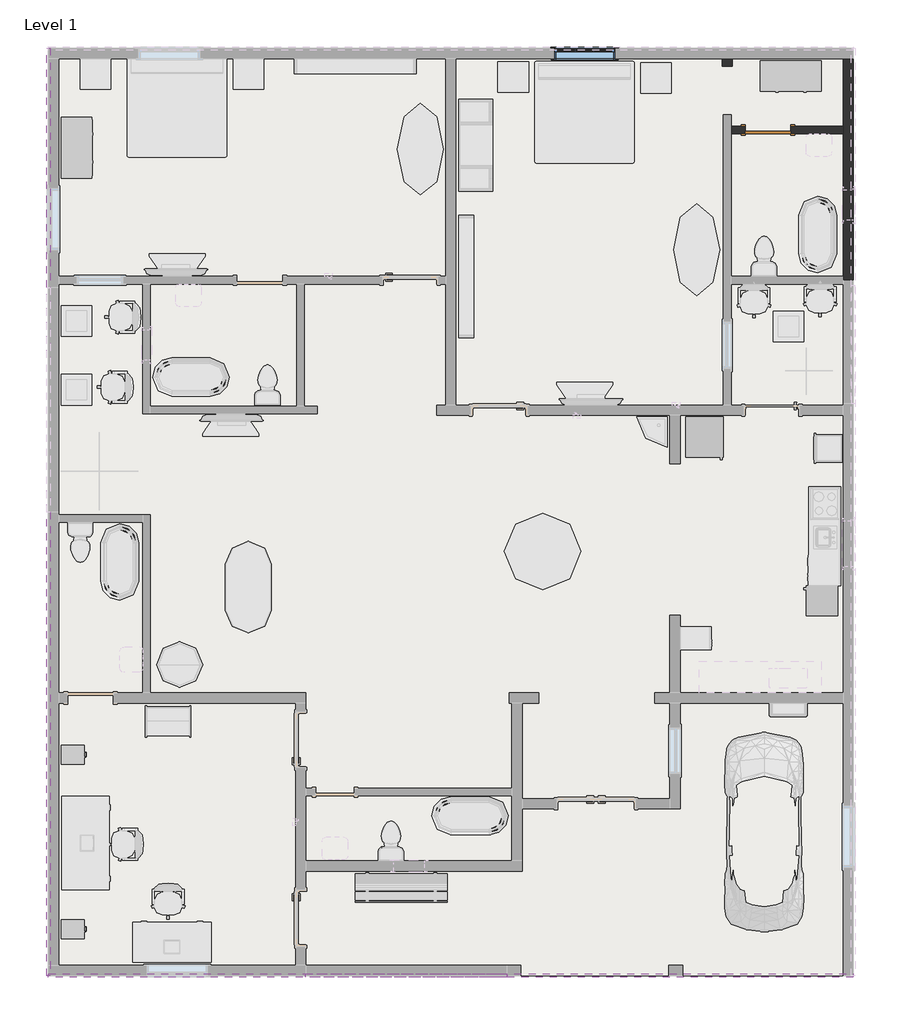
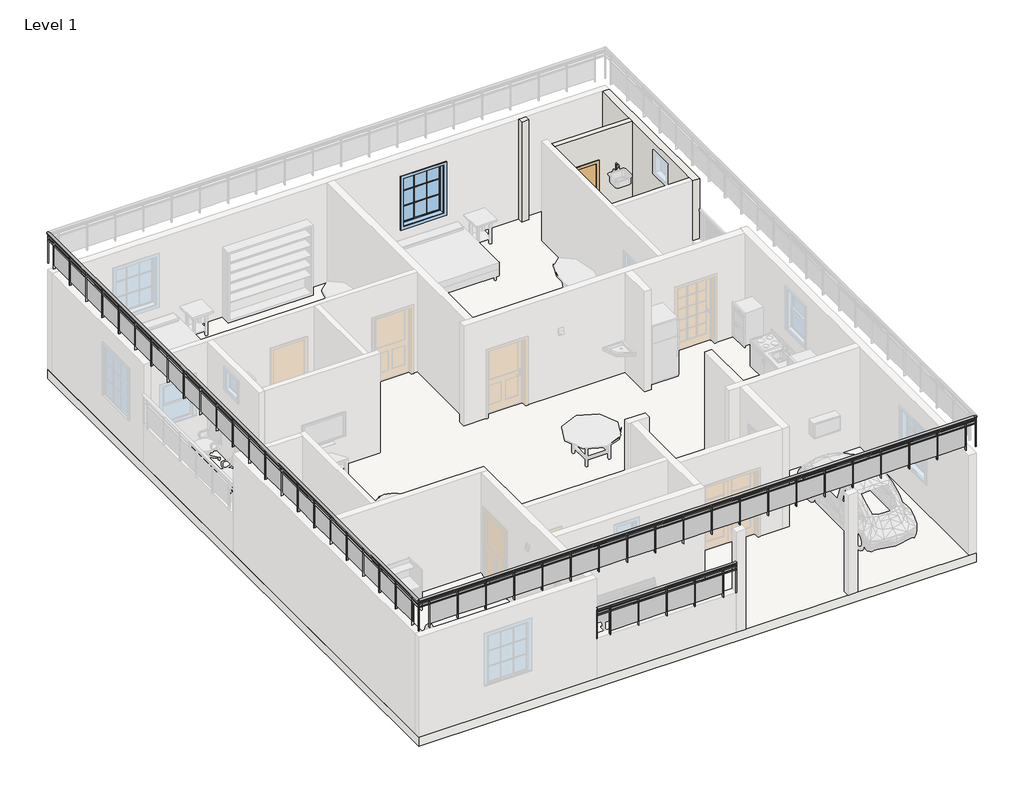
# One storey, part 2 of 4: 3 railings, 3 walls, 1 door, 1 slab, 1 window.
"""IFC4 building model written with IfcOpenShell, lengths in millimetres."""

from ifc_helpers import new_model, si_unit, point, frame, origin, origin_with_axes, place, context, project, spatial, polyline, ellipse_curve, trimmed, outline, extrude, faceted_brep, transform, mapped, element, save
from ifc_brep_helpers import plane_surface, extruded_surface, advanced_brep
from components import door_16372e1c, window_cfa1ffdd

model = new_model("IFC4")

# Units and contexts
model_context = context("Model", 3, world=origin())
ifc_project = project(units=[si_unit("LENGTHUNIT", "METRE", prefix="MILLI")], contexts=[model_context])

# Site, building, storey
site = spatial("IfcSite", under=ifc_project)
building = spatial("IfcBuilding", under=site)
storey = spatial("IfcBuildingStorey", under=building, Name="Level 1", Elevation=0.0)

# Door
placement = place(None, origin())
door_shape = door_16372e1c(model_context)
element("IfcDoor", 1, ObjectType="Single-Flush : 36\" x 84\"", at=placement, inside=storey, context=model_context, shape_type="MappedRepresentation", body=[
    mapped(door_shape, transform((-3290.7484731, 10947.0442281, 0.0), x_axis=(-1.0, 0.0, 0.0), y_axis=(0.0, -1.0, 0.0), z_axis=(0.0, 0.0, 1.0))),
])

# Railings
element("IfcRailing", 2, ObjectType="Glass Panel - Bottom Fill", at=placement, inside=storey, context=model_context, shape_type="SolidModel", body=[
    advanced_brep(
    [(-17603.6484731, 12572.6442281, 4165.6), (-17679.8484731, 12572.6442281, 4165.6), (-17603.6484731, -5918.5557719, 4165.6), (-17679.8484731, -5918.5557719, 4165.6)],
    [
        (0, 1, ellipse_curve(frame((-17641.7484731, 12572.6442281, 4165.6), z_axis=(0.0, 1.0, 0.0), x_axis=(-1.0, 0.0, 0.0)), 38.1, 28.575)),
        (1, 0, ellipse_curve(frame((-17641.7484731, 12572.6442281, 4165.6), z_axis=(0.0, 1.0, 0.0), x_axis=(-1.0, 0.0, 0.0)), 38.1, 28.575)),
        (2, 3, ellipse_curve(frame((-17641.7484731, -5918.5557719, 4165.6), z_axis=(0.0, -1.0, 0.0), x_axis=(-1.0, 0.0, 0.0)), 38.1, 28.575)),
        (3, 2, ellipse_curve(frame((-17641.7484731, -5918.5557719, 4165.6), z_axis=(0.0, -1.0, 0.0), x_axis=(-1.0, 0.0, 0.0)), 38.1, 28.575)),
        (0, 2),
        (3, 1),
    ],
    [
        plane_surface(frame((-17641.7484731, 12572.6442281, 4165.6), z_axis=(0.0, 1.0, 0.0), x_axis=(0.0, 0.0, -1.0))),
        plane_surface(frame((-17641.7484731, -5918.5557719, 4165.6), z_axis=(0.0, -1.0, 0.0), x_axis=(0.0, 0.0, -1.0))),
        extruded_surface(trimmed(ellipse_curve(frame((-17641.7484731, -5918.5557719, 4165.6), z_axis=(0.0, 1.0, 0.0), x_axis=(-1.0, 0.0, 0.0)), 38.1, 28.575), [point((-17603.6484731, -5918.5557719, 4165.6))], [point((-17679.8484731, -5918.5557719, 4165.6))], True, "CARTESIAN"), (0.0, 18491.2, 0.0), 18491.2),
        extruded_surface(trimmed(ellipse_curve(frame((-17641.7484731, -5918.5557719, 4165.6), z_axis=(0.0, 1.0, 0.0), x_axis=(-1.0, 0.0, 0.0)), 38.1, 28.575), [point((-17679.8484731, -5918.5557719, 4165.6))], [point((-17603.6484731, -5918.5557719, 4165.6))], True, "CARTESIAN"), (0.0, 18491.2, 0.0), 18491.2),
    ],
    [
        (0, [[1, 2]]),
        (1, [[3, 4]]),
        (2, [[-1, 5, -4, 6]]),
        (3, [[-2, -6, -3, -5]]),
    ],
),
    extrude(outline(polyline([(-17654.4484731, 12572.6442281), (-17629.0484731, 12572.6442281), (-17629.0484731, -5918.5557719), (-17654.4484731, -5918.5557719), (-17654.4484731, 12572.6442281)])), frame((0.0, 0.0, 4051.3), z_axis=(0.0, 0.0, 1.0), x_axis=(1.0, 0.0, 0.0)), (0.0, 0.0, 1.0), 25.4),
    extrude(outline(polyline([(-17654.4484731, 12572.6442281), (-17629.0484731, 12572.6442281), (-17629.0484731, -5918.5557719), (-17654.4484731, -5918.5557719), (-17654.4484731, 12572.6442281)])), frame((0.0, 0.0, 3949.7), z_axis=(0.0, 0.0, 1.0), x_axis=(1.0, 0.0, 0.0)), (0.0, 0.0, 1.0), 25.4),
    extrude(outline(polyline([(-17667.1484731, -5607.4057719), (-17616.3484731, -5607.4057719), (-17616.3484731, -5620.1057719), (-17667.1484731, -5620.1057719), (-17667.1484731, -5607.4057719)])), frame((0.0, 0.0, 3251.2), z_axis=(0.0, 0.0, 1.0), x_axis=(1.0, 0.0, 0.0)), (0.0, 0.0, 1.0), 885.6788223),
    extrude(outline(polyline([(-17635.2133161, -4800.9557719), (-17635.2133161, -5613.7557719), (-17641.5633161, -5613.7557719), (-17641.5633161, -4800.9557719), (-17635.2133161, -4800.9557719)])), frame((0.0, 0.0, 3352.8), z_axis=(0.0, 0.0, 1.0), x_axis=(1.0, 0.0, 0.0)), (0.0, 0.0, 1.0), 596.9),
    extrude(outline(polyline([(-17667.1484731, -4794.6057719), (-17616.3484731, -4794.6057719), (-17616.3484731, -4807.3057719), (-17667.1484731, -4807.3057719), (-17667.1484731, -4794.6057719)])), frame((0.0, 0.0, 3251.2), z_axis=(0.0, 0.0, 1.0), x_axis=(1.0, 0.0, 0.0)), (0.0, 0.0, 1.0), 885.6788223),
    extrude(outline(polyline([(-17635.2133161, -3988.1557719), (-17635.2133161, -4800.9557719), (-17641.5633161, -4800.9557719), (-17641.5633161, -3988.1557719), (-17635.2133161, -3988.1557719)])), frame((0.0, 0.0, 3352.8), z_axis=(0.0, 0.0, 1.0), x_axis=(1.0, 0.0, 0.0)), (0.0, 0.0, 1.0), 596.9),
    extrude(outline(polyline([(-17667.1484731, -3981.8057719), (-17616.3484731, -3981.8057719), (-17616.3484731, -3994.5057719), (-17667.1484731, -3994.5057719), (-17667.1484731, -3981.8057719)])), frame((0.0, 0.0, 3251.2), z_axis=(0.0, 0.0, 1.0), x_axis=(1.0, 0.0, 0.0)), (0.0, 0.0, 1.0), 885.6788223),
    extrude(outline(polyline([(-17635.2133161, -3175.3557719), (-17635.2133161, -3988.1557719), (-17641.5633161, -3988.1557719), (-17641.5633161, -3175.3557719), (-17635.2133161, -3175.3557719)])), frame((0.0, 0.0, 3352.8), z_axis=(0.0, 0.0, 1.0), x_axis=(1.0, 0.0, 0.0)), (0.0, 0.0, 1.0), 596.9),
    extrude(outline(polyline([(-17667.1484731, -3169.0057719), (-17616.3484731, -3169.0057719), (-17616.3484731, -3181.7057719), (-17667.1484731, -3181.7057719), (-17667.1484731, -3169.0057719)])), frame((0.0, 0.0, 3251.2), z_axis=(0.0, 0.0, 1.0), x_axis=(1.0, 0.0, 0.0)), (0.0, 0.0, 1.0), 885.6788223),
    extrude(outline(polyline([(-17635.2133161, -2362.5557719), (-17635.2133161, -3175.3557719), (-17641.5633161, -3175.3557719), (-17641.5633161, -2362.5557719), (-17635.2133161, -2362.5557719)])), frame((0.0, 0.0, 3352.8), z_axis=(0.0, 0.0, 1.0), x_axis=(1.0, 0.0, 0.0)), (0.0, 0.0, 1.0), 596.9),
    extrude(outline(polyline([(-17667.1484731, -2356.2057719), (-17616.3484731, -2356.2057719), (-17616.3484731, -2368.9057719), (-17667.1484731, -2368.9057719), (-17667.1484731, -2356.2057719)])), frame((0.0, 0.0, 3251.2), z_axis=(0.0, 0.0, 1.0), x_axis=(1.0, 0.0, 0.0)), (0.0, 0.0, 1.0), 885.6788223),
    extrude(outline(polyline([(-17635.2133161, -1549.7557719), (-17635.2133161, -2362.5557719), (-17641.5633161, -2362.5557719), (-17641.5633161, -1549.7557719), (-17635.2133161, -1549.7557719)])), frame((0.0, 0.0, 3352.8), z_axis=(0.0, 0.0, 1.0), x_axis=(1.0, 0.0, 0.0)), (0.0, 0.0, 1.0), 596.9),
    extrude(outline(polyline([(-17667.1484731, -1543.4057719), (-17616.3484731, -1543.4057719), (-17616.3484731, -1556.1057719), (-17667.1484731, -1556.1057719), (-17667.1484731, -1543.4057719)])), frame((0.0, 0.0, 3251.2), z_axis=(0.0, 0.0, 1.0), x_axis=(1.0, 0.0, 0.0)), (0.0, 0.0, 1.0), 885.6788223),
    extrude(outline(polyline([(-17635.2133161, -736.9557719), (-17635.2133161, -1549.7557719), (-17641.5633161, -1549.7557719), (-17641.5633161, -736.9557719), (-17635.2133161, -736.9557719)])), frame((0.0, 0.0, 3352.8), z_axis=(0.0, 0.0, 1.0), x_axis=(1.0, 0.0, 0.0)), (0.0, 0.0, 1.0), 596.9),
    extrude(outline(polyline([(-17667.1484731, -730.6057719), (-17616.3484731, -730.6057719), (-17616.3484731, -743.3057719), (-17667.1484731, -743.3057719), (-17667.1484731, -730.6057719)])), frame((0.0, 0.0, 3251.2), z_axis=(0.0, 0.0, 1.0), x_axis=(1.0, 0.0, 0.0)), (0.0, 0.0, 1.0), 885.6788223),
    extrude(outline(polyline([(-17635.2133161, 75.8442281), (-17635.2133161, -736.9557719), (-17641.5633161, -736.9557719), (-17641.5633161, 75.8442281), (-17635.2133161, 75.8442281)])), frame((0.0, 0.0, 3352.8), z_axis=(0.0, 0.0, 1.0), x_axis=(1.0, 0.0, 0.0)), (0.0, 0.0, 1.0), 596.9),
    extrude(outline(polyline([(-17667.1484731, 82.1942281), (-17616.3484731, 82.1942281), (-17616.3484731, 69.4942281), (-17667.1484731, 69.4942281), (-17667.1484731, 82.1942281)])), frame((0.0, 0.0, 3251.2), z_axis=(0.0, 0.0, 1.0), x_axis=(1.0, 0.0, 0.0)), (0.0, 0.0, 1.0), 885.6788223),
    extrude(outline(polyline([(-17635.2133161, 888.6442281), (-17635.2133161, 75.8442281), (-17641.5633161, 75.8442281), (-17641.5633161, 888.6442281), (-17635.2133161, 888.6442281)])), frame((0.0, 0.0, 3352.8), z_axis=(0.0, 0.0, 1.0), x_axis=(1.0, 0.0, 0.0)), (0.0, 0.0, 1.0), 596.9),
    extrude(outline(polyline([(-17667.1484731, 894.9942281), (-17616.3484731, 894.9942281), (-17616.3484731, 882.2942281), (-17667.1484731, 882.2942281), (-17667.1484731, 894.9942281)])), frame((0.0, 0.0, 3251.2), z_axis=(0.0, 0.0, 1.0), x_axis=(1.0, 0.0, 0.0)), (0.0, 0.0, 1.0), 885.6788223),
    extrude(outline(polyline([(-17635.2133161, 1701.4442281), (-17635.2133161, 888.6442281), (-17641.5633161, 888.6442281), (-17641.5633161, 1701.4442281), (-17635.2133161, 1701.4442281)])), frame((0.0, 0.0, 3352.8), z_axis=(0.0, 0.0, 1.0), x_axis=(1.0, 0.0, 0.0)), (0.0, 0.0, 1.0), 596.9),
    extrude(outline(polyline([(-17667.1484731, 1707.7942281), (-17616.3484731, 1707.7942281), (-17616.3484731, 1695.0942281), (-17667.1484731, 1695.0942281), (-17667.1484731, 1707.7942281)])), frame((0.0, 0.0, 3251.2), z_axis=(0.0, 0.0, 1.0), x_axis=(1.0, 0.0, 0.0)), (0.0, 0.0, 1.0), 885.6788223),
    extrude(outline(polyline([(-17635.2133161, 2514.2442281), (-17635.2133161, 1701.4442281), (-17641.5633161, 1701.4442281), (-17641.5633161, 2514.2442281), (-17635.2133161, 2514.2442281)])), frame((0.0, 0.0, 3352.8), z_axis=(0.0, 0.0, 1.0), x_axis=(1.0, 0.0, 0.0)), (0.0, 0.0, 1.0), 596.9),
    extrude(outline(polyline([(-17667.1484731, 2520.5942281), (-17616.3484731, 2520.5942281), (-17616.3484731, 2507.8942281), (-17667.1484731, 2507.8942281), (-17667.1484731, 2520.5942281)])), frame((0.0, 0.0, 3251.2), z_axis=(0.0, 0.0, 1.0), x_axis=(1.0, 0.0, 0.0)), (0.0, 0.0, 1.0), 885.6788223),
    extrude(outline(polyline([(-17635.2133161, 3327.0442281), (-17635.2133161, 2514.2442281), (-17641.5633161, 2514.2442281), (-17641.5633161, 3327.0442281), (-17635.2133161, 3327.0442281)])), frame((0.0, 0.0, 3352.8), z_axis=(0.0, 0.0, 1.0), x_axis=(1.0, 0.0, 0.0)), (0.0, 0.0, 1.0), 596.9),
    extrude(outline(polyline([(-17667.1484731, 3333.3942281), (-17616.3484731, 3333.3942281), (-17616.3484731, 3320.6942281), (-17667.1484731, 3320.6942281), (-17667.1484731, 3333.3942281)])), frame((0.0, 0.0, 3251.2), z_axis=(0.0, 0.0, 1.0), x_axis=(1.0, 0.0, 0.0)), (0.0, 0.0, 1.0), 885.6788223),
    extrude(outline(polyline([(-17635.2133161, 4139.8442281), (-17635.2133161, 3327.0442281), (-17641.5633161, 3327.0442281), (-17641.5633161, 4139.8442281), (-17635.2133161, 4139.8442281)])), frame((0.0, 0.0, 3352.8), z_axis=(0.0, 0.0, 1.0), x_axis=(1.0, 0.0, 0.0)), (0.0, 0.0, 1.0), 596.9),
    extrude(outline(polyline([(-17667.1484731, 4146.1942281), (-17616.3484731, 4146.1942281), (-17616.3484731, 4133.4942281), (-17667.1484731, 4133.4942281), (-17667.1484731, 4146.1942281)])), frame((0.0, 0.0, 3251.2), z_axis=(0.0, 0.0, 1.0), x_axis=(1.0, 0.0, 0.0)), (0.0, 0.0, 1.0), 885.6788223),
    extrude(outline(polyline([(-17635.2133161, 4952.6442281), (-17635.2133161, 4139.8442281), (-17641.5633161, 4139.8442281), (-17641.5633161, 4952.6442281), (-17635.2133161, 4952.6442281)])), frame((0.0, 0.0, 3352.8), z_axis=(0.0, 0.0, 1.0), x_axis=(1.0, 0.0, 0.0)), (0.0, 0.0, 1.0), 596.9),
    extrude(outline(polyline([(-17667.1484731, 4958.9942281), (-17616.3484731, 4958.9942281), (-17616.3484731, 4946.2942281), (-17667.1484731, 4946.2942281), (-17667.1484731, 4958.9942281)])), frame((0.0, 0.0, 3251.2), z_axis=(0.0, 0.0, 1.0), x_axis=(1.0, 0.0, 0.0)), (0.0, 0.0, 1.0), 885.6788223),
    extrude(outline(polyline([(-17635.2133161, 5765.4442281), (-17635.2133161, 4952.6442281), (-17641.5633161, 4952.6442281), (-17641.5633161, 5765.4442281), (-17635.2133161, 5765.4442281)])), frame((0.0, 0.0, 3352.8), z_axis=(0.0, 0.0, 1.0), x_axis=(1.0, 0.0, 0.0)), (0.0, 0.0, 1.0), 596.9),
    extrude(outline(polyline([(-17667.1484731, 5771.7942281), (-17616.3484731, 5771.7942281), (-17616.3484731, 5759.0942281), (-17667.1484731, 5759.0942281), (-17667.1484731, 5771.7942281)])), frame((0.0, 0.0, 3251.2), z_axis=(0.0, 0.0, 1.0), x_axis=(1.0, 0.0, 0.0)), (0.0, 0.0, 1.0), 885.6788223),
    extrude(outline(polyline([(-17635.2133161, 6578.2442281), (-17635.2133161, 5765.4442281), (-17641.5633161, 5765.4442281), (-17641.5633161, 6578.2442281), (-17635.2133161, 6578.2442281)])), frame((0.0, 0.0, 3352.8), z_axis=(0.0, 0.0, 1.0), x_axis=(1.0, 0.0, 0.0)), (0.0, 0.0, 1.0), 596.9),
    extrude(outline(polyline([(-17667.1484731, 6584.5942281), (-17616.3484731, 6584.5942281), (-17616.3484731, 6571.8942281), (-17667.1484731, 6571.8942281), (-17667.1484731, 6584.5942281)])), frame((0.0, 0.0, 3251.2), z_axis=(0.0, 0.0, 1.0), x_axis=(1.0, 0.0, 0.0)), (0.0, 0.0, 1.0), 885.6788223),
    extrude(outline(polyline([(-17635.2133161, 7391.0442281), (-17635.2133161, 6578.2442281), (-17641.5633161, 6578.2442281), (-17641.5633161, 7391.0442281), (-17635.2133161, 7391.0442281)])), frame((0.0, 0.0, 3352.8), z_axis=(0.0, 0.0, 1.0), x_axis=(1.0, 0.0, 0.0)), (0.0, 0.0, 1.0), 596.9),
    extrude(outline(polyline([(-17667.1484731, 7397.3942281), (-17616.3484731, 7397.3942281), (-17616.3484731, 7384.6942281), (-17667.1484731, 7384.6942281), (-17667.1484731, 7397.3942281)])), frame((0.0, 0.0, 3251.2), z_axis=(0.0, 0.0, 1.0), x_axis=(1.0, 0.0, 0.0)), (0.0, 0.0, 1.0), 885.6788223),
    extrude(outline(polyline([(-17635.2133161, 8203.8442281), (-17635.2133161, 7391.0442281), (-17641.5633161, 7391.0442281), (-17641.5633161, 8203.8442281), (-17635.2133161, 8203.8442281)])), frame((0.0, 0.0, 3352.8), z_axis=(0.0, 0.0, 1.0), x_axis=(1.0, 0.0, 0.0)), (0.0, 0.0, 1.0), 596.9),
    extrude(outline(polyline([(-17667.1484731, 8210.1942281), (-17616.3484731, 8210.1942281), (-17616.3484731, 8197.4942281), (-17667.1484731, 8197.4942281), (-17667.1484731, 8210.1942281)])), frame((0.0, 0.0, 3251.2), z_axis=(0.0, 0.0, 1.0), x_axis=(1.0, 0.0, 0.0)), (0.0, 0.0, 1.0), 885.6788223),
    extrude(outline(polyline([(-17635.2133161, 9016.6442281), (-17635.2133161, 8203.8442281), (-17641.5633161, 8203.8442281), (-17641.5633161, 9016.6442281), (-17635.2133161, 9016.6442281)])), frame((0.0, 0.0, 3352.8), z_axis=(0.0, 0.0, 1.0), x_axis=(1.0, 0.0, 0.0)), (0.0, 0.0, 1.0), 596.9),
    extrude(outline(polyline([(-17667.1484731, 9022.9942281), (-17616.3484731, 9022.9942281), (-17616.3484731, 9010.2942281), (-17667.1484731, 9010.2942281), (-17667.1484731, 9022.9942281)])), frame((0.0, 0.0, 3251.2), z_axis=(0.0, 0.0, 1.0), x_axis=(1.0, 0.0, 0.0)), (0.0, 0.0, 1.0), 885.6788223),
    extrude(outline(polyline([(-17635.2133161, 9829.4442281), (-17635.2133161, 9016.6442281), (-17641.5633161, 9016.6442281), (-17641.5633161, 9829.4442281), (-17635.2133161, 9829.4442281)])), frame((0.0, 0.0, 3352.8), z_axis=(0.0, 0.0, 1.0), x_axis=(1.0, 0.0, 0.0)), (0.0, 0.0, 1.0), 596.9),
    extrude(outline(polyline([(-17667.1484731, 9835.7942281), (-17616.3484731, 9835.7942281), (-17616.3484731, 9823.0942281), (-17667.1484731, 9823.0942281), (-17667.1484731, 9835.7942281)])), frame((0.0, 0.0, 3251.2), z_axis=(0.0, 0.0, 1.0), x_axis=(1.0, 0.0, 0.0)), (0.0, 0.0, 1.0), 885.6788223),
    extrude(outline(polyline([(-17635.2133161, 10642.2442281), (-17635.2133161, 9829.4442281), (-17641.5633161, 9829.4442281), (-17641.5633161, 10642.2442281), (-17635.2133161, 10642.2442281)])), frame((0.0, 0.0, 3352.8), z_axis=(0.0, 0.0, 1.0), x_axis=(1.0, 0.0, 0.0)), (0.0, 0.0, 1.0), 596.9),
    extrude(outline(polyline([(-17667.1484731, 10648.5942281), (-17616.3484731, 10648.5942281), (-17616.3484731, 10635.8942281), (-17667.1484731, 10635.8942281), (-17667.1484731, 10648.5942281)])), frame((0.0, 0.0, 3251.2), z_axis=(0.0, 0.0, 1.0), x_axis=(1.0, 0.0, 0.0)), (0.0, 0.0, 1.0), 885.6788223),
    extrude(outline(polyline([(-17635.2133161, 11455.0442281), (-17635.2133161, 10642.2442281), (-17641.5633161, 10642.2442281), (-17641.5633161, 11455.0442281), (-17635.2133161, 11455.0442281)])), frame((0.0, 0.0, 3352.8), z_axis=(0.0, 0.0, 1.0), x_axis=(1.0, 0.0, 0.0)), (0.0, 0.0, 1.0), 596.9),
    extrude(outline(polyline([(-17667.1484731, 11461.3942281), (-17616.3484731, 11461.3942281), (-17616.3484731, 11448.6942281), (-17667.1484731, 11448.6942281), (-17667.1484731, 11461.3942281)])), frame((0.0, 0.0, 3251.2), z_axis=(0.0, 0.0, 1.0), x_axis=(1.0, 0.0, 0.0)), (0.0, 0.0, 1.0), 885.6788223),
    extrude(outline(polyline([(-17635.2133161, 12267.8442281), (-17635.2133161, 11455.0442281), (-17641.5633161, 11455.0442281), (-17641.5633161, 12267.8442281), (-17635.2133161, 12267.8442281)])), frame((0.0, 0.0, 3352.8), z_axis=(0.0, 0.0, 1.0), x_axis=(1.0, 0.0, 0.0)), (0.0, 0.0, 1.0), 596.9),
    extrude(outline(polyline([(-17667.1484731, 12274.1942281), (-17616.3484731, 12274.1942281), (-17616.3484731, 12261.4942281), (-17667.1484731, 12261.4942281), (-17667.1484731, 12274.1942281)])), frame((0.0, 0.0, 3251.2), z_axis=(0.0, 0.0, 1.0), x_axis=(1.0, 0.0, 0.0)), (0.0, 0.0, 1.0), 885.6788223),
    extrude(outline(polyline([(-17651.2734731, -5905.8557719), (-17632.2234731, -5905.8557719), (-17632.2234731, -5924.9057719), (-17651.2734731, -5924.9057719), (-17651.2734731, -5905.8557719)])), frame((0.0, 0.0, 3251.2), z_axis=(0.0, 0.0, 1.0), x_axis=(1.0, 0.0, 0.0)), (0.0, 0.0, 1.0), 885.6788223),
    extrude(outline(polyline([(-17651.2734731, 12578.9942281), (-17632.2234731, 12578.9942281), (-17632.2234731, 12559.9442281), (-17651.2734731, 12559.9442281), (-17651.2734731, 12578.9942281)])), frame((0.0, 0.0, 3251.2), z_axis=(0.0, 0.0, 1.0), x_axis=(1.0, 0.0, 0.0)), (0.0, 0.0, 1.0), 885.6788223),
])
element("IfcRailing", 3, ObjectType="Glass Panel - Bottom Fill", at=placement, inside=storey, context=model_context, shape_type="SolidModel", body=[
    advanced_brep(
    [(-17641.7484731, -5880.4557719, 4165.6), (-17641.7484731, -5956.6557719, 4165.6), (-1588.9484731, -5880.4557719, 4165.6), (-1588.9484731, -5956.6557719, 4165.6)],
    [
        (0, 1, ellipse_curve(frame((-17641.7484731, -5918.5557719, 4165.6), z_axis=(-1.0, 0.0, 0.0), x_axis=(0.0, -1.0, 0.0)), 38.1, 28.575)),
        (1, 0, ellipse_curve(frame((-17641.7484731, -5918.5557719, 4165.6), z_axis=(-1.0, 0.0, 0.0), x_axis=(0.0, -1.0, 0.0)), 38.1, 28.575)),
        (2, 3, ellipse_curve(frame((-1588.9484731, -5918.5557719, 4165.6), z_axis=(1.0, 0.0, 0.0), x_axis=(0.0, -1.0, 0.0)), 38.1, 28.575)),
        (3, 2, ellipse_curve(frame((-1588.9484731, -5918.5557719, 4165.6), z_axis=(1.0, 0.0, 0.0), x_axis=(0.0, -1.0, 0.0)), 38.1, 28.575)),
        (0, 2),
        (3, 1),
    ],
    [
        plane_surface(frame((-17641.7484731, -5918.5557719, 4165.6), z_axis=(-1.0, 0.0, 0.0), x_axis=(0.0, 1.0, 0.0))),
        plane_surface(frame((-1588.9484731, -5918.5557719, 4165.6), z_axis=(1.0, 0.0, 0.0), x_axis=(0.0, 1.0, 0.0))),
        extruded_surface(trimmed(ellipse_curve(frame((-1588.9484731, -5918.5557719, 4165.6), z_axis=(-1.0, 0.0, 0.0), x_axis=(0.0, -1.0, 0.0)), 38.1, 28.575), [point((-1588.9484731, -5880.4557719, 4165.6))], [point((-1588.9484731, -5956.6557719, 4165.6))], True, "CARTESIAN"), (-16052.800000000001, 0.0, 0.0), 16052.800000000001),
        extruded_surface(trimmed(ellipse_curve(frame((-1588.9484731, -5918.5557719, 4165.6), z_axis=(-1.0, 0.0, 0.0), x_axis=(0.0, -1.0, 0.0)), 38.1, 28.575), [point((-1588.9484731, -5956.6557719, 4165.6))], [point((-1588.9484731, -5880.4557719, 4165.6))], True, "CARTESIAN"), (-16052.800000000001, 0.0, 0.0), 16052.800000000001),
    ],
    [
        (0, [[1, 2]]),
        (1, [[3, 4]]),
        (2, [[-1, 5, -4, 6]]),
        (3, [[-2, -6, -3, -5]]),
    ],
),
    extrude(outline(polyline([(-17641.7484731, -5931.2557719), (-17641.7484731, -5905.8557719), (-1588.9484731, -5905.8557719), (-1588.9484731, -5931.2557719), (-17641.7484731, -5931.2557719)])), frame((0.0, 0.0, 4051.3), z_axis=(0.0, 0.0, 1.0), x_axis=(1.0, 0.0, 0.0)), (0.0, 0.0, 1.0), 25.4),
    extrude(outline(polyline([(-17641.7484731, -5931.2557719), (-17641.7484731, -5905.8557719), (-1588.9484731, -5905.8557719), (-1588.9484731, -5931.2557719), (-17641.7484731, -5931.2557719)])), frame((0.0, 0.0, 3949.7), z_axis=(0.0, 0.0, 1.0), x_axis=(1.0, 0.0, 0.0)), (0.0, 0.0, 1.0), 25.4),
    extrude(outline(polyline([(-1900.0984731, -5943.9557719), (-1900.0984731, -5893.1557719), (-1887.3984731, -5893.1557719), (-1887.3984731, -5943.9557719), (-1900.0984731, -5943.9557719)])), frame((0.0, 0.0, 3251.2), z_axis=(0.0, 0.0, 1.0), x_axis=(1.0, 0.0, 0.0)), (0.0, 0.0, 1.0), 885.6788223),
    extrude(outline(polyline([(-2706.5484731, -5912.0206149), (-1893.7484731, -5912.0206149), (-1893.7484731, -5918.3706149), (-2706.5484731, -5918.3706149), (-2706.5484731, -5912.0206149)])), frame((0.0, 0.0, 3352.8), z_axis=(0.0, 0.0, 1.0), x_axis=(1.0, 0.0, 0.0)), (0.0, 0.0, 1.0), 596.9),
    extrude(outline(polyline([(-2712.8984731, -5943.9557719), (-2712.8984731, -5893.1557719), (-2700.1984731, -5893.1557719), (-2700.1984731, -5943.9557719), (-2712.8984731, -5943.9557719)])), frame((0.0, 0.0, 3251.2), z_axis=(0.0, 0.0, 1.0), x_axis=(1.0, 0.0, 0.0)), (0.0, 0.0, 1.0), 885.6788223),
    extrude(outline(polyline([(-3519.3484731, -5912.0206149), (-2706.5484731, -5912.0206149), (-2706.5484731, -5918.3706149), (-3519.3484731, -5918.3706149), (-3519.3484731, -5912.0206149)])), frame((0.0, 0.0, 3352.8), z_axis=(0.0, 0.0, 1.0), x_axis=(1.0, 0.0, 0.0)), (0.0, 0.0, 1.0), 596.9),
    extrude(outline(polyline([(-3525.6984731, -5943.9557719), (-3525.6984731, -5893.1557719), (-3512.9984731, -5893.1557719), (-3512.9984731, -5943.9557719), (-3525.6984731, -5943.9557719)])), frame((0.0, 0.0, 3251.2), z_axis=(0.0, 0.0, 1.0), x_axis=(1.0, 0.0, 0.0)), (0.0, 0.0, 1.0), 885.6788223),
    extrude(outline(polyline([(-4332.1484731, -5912.0206149), (-3519.3484731, -5912.0206149), (-3519.3484731, -5918.3706149), (-4332.1484731, -5918.3706149), (-4332.1484731, -5912.0206149)])), frame((0.0, 0.0, 3352.8), z_axis=(0.0, 0.0, 1.0), x_axis=(1.0, 0.0, 0.0)), (0.0, 0.0, 1.0), 596.9),
    extrude(outline(polyline([(-4338.4984731, -5943.9557719), (-4338.4984731, -5893.1557719), (-4325.7984731, -5893.1557719), (-4325.7984731, -5943.9557719), (-4338.4984731, -5943.9557719)])), frame((0.0, 0.0, 3251.2), z_axis=(0.0, 0.0, 1.0), x_axis=(1.0, 0.0, 0.0)), (0.0, 0.0, 1.0), 885.6788223),
    extrude(outline(polyline([(-5144.9484731, -5912.0206149), (-4332.1484731, -5912.0206149), (-4332.1484731, -5918.3706149), (-5144.9484731, -5918.3706149), (-5144.9484731, -5912.0206149)])), frame((0.0, 0.0, 3352.8), z_axis=(0.0, 0.0, 1.0), x_axis=(1.0, 0.0, 0.0)), (0.0, 0.0, 1.0), 596.9),
    extrude(outline(polyline([(-5151.2984731, -5943.9557719), (-5151.2984731, -5893.1557719), (-5138.5984731, -5893.1557719), (-5138.5984731, -5943.9557719), (-5151.2984731, -5943.9557719)])), frame((0.0, 0.0, 3251.2), z_axis=(0.0, 0.0, 1.0), x_axis=(1.0, 0.0, 0.0)), (0.0, 0.0, 1.0), 885.6788223),
    extrude(outline(polyline([(-5957.7484731, -5912.0206149), (-5144.9484731, -5912.0206149), (-5144.9484731, -5918.3706149), (-5957.7484731, -5918.3706149), (-5957.7484731, -5912.0206149)])), frame((0.0, 0.0, 3352.8), z_axis=(0.0, 0.0, 1.0), x_axis=(1.0, 0.0, 0.0)), (0.0, 0.0, 1.0), 596.9),
    extrude(outline(polyline([(-5964.0984731, -5943.9557719), (-5964.0984731, -5893.1557719), (-5951.3984731, -5893.1557719), (-5951.3984731, -5943.9557719), (-5964.0984731, -5943.9557719)])), frame((0.0, 0.0, 3251.2), z_axis=(0.0, 0.0, 1.0), x_axis=(1.0, 0.0, 0.0)), (0.0, 0.0, 1.0), 885.6788223),
    extrude(outline(polyline([(-6770.5484731, -5912.0206149), (-5957.7484731, -5912.0206149), (-5957.7484731, -5918.3706149), (-6770.5484731, -5918.3706149), (-6770.5484731, -5912.0206149)])), frame((0.0, 0.0, 3352.8), z_axis=(0.0, 0.0, 1.0), x_axis=(1.0, 0.0, 0.0)), (0.0, 0.0, 1.0), 596.9),
    extrude(outline(polyline([(-6776.8984731, -5943.9557719), (-6776.8984731, -5893.1557719), (-6764.1984731, -5893.1557719), (-6764.1984731, -5943.9557719), (-6776.8984731, -5943.9557719)])), frame((0.0, 0.0, 3251.2), z_axis=(0.0, 0.0, 1.0), x_axis=(1.0, 0.0, 0.0)), (0.0, 0.0, 1.0), 885.6788223),
    extrude(outline(polyline([(-7583.3484731, -5912.0206149), (-6770.5484731, -5912.0206149), (-6770.5484731, -5918.3706149), (-7583.3484731, -5918.3706149), (-7583.3484731, -5912.0206149)])), frame((0.0, 0.0, 3352.8), z_axis=(0.0, 0.0, 1.0), x_axis=(1.0, 0.0, 0.0)), (0.0, 0.0, 1.0), 596.9),
    extrude(outline(polyline([(-7589.6984731, -5943.9557719), (-7589.6984731, -5893.1557719), (-7576.9984731, -5893.1557719), (-7576.9984731, -5943.9557719), (-7589.6984731, -5943.9557719)])), frame((0.0, 0.0, 3251.2), z_axis=(0.0, 0.0, 1.0), x_axis=(1.0, 0.0, 0.0)), (0.0, 0.0, 1.0), 885.6788223),
    extrude(outline(polyline([(-8396.1484731, -5912.0206149), (-7583.3484731, -5912.0206149), (-7583.3484731, -5918.3706149), (-8396.1484731, -5918.3706149), (-8396.1484731, -5912.0206149)])), frame((0.0, 0.0, 3352.8), z_axis=(0.0, 0.0, 1.0), x_axis=(1.0, 0.0, 0.0)), (0.0, 0.0, 1.0), 596.9),
    extrude(outline(polyline([(-8402.4984731, -5943.9557719), (-8402.4984731, -5893.1557719), (-8389.7984731, -5893.1557719), (-8389.7984731, -5943.9557719), (-8402.4984731, -5943.9557719)])), frame((0.0, 0.0, 3251.2), z_axis=(0.0, 0.0, 1.0), x_axis=(1.0, 0.0, 0.0)), (0.0, 0.0, 1.0), 885.6788223),
    extrude(outline(polyline([(-9208.9484731, -5912.0206149), (-8396.1484731, -5912.0206149), (-8396.1484731, -5918.3706149), (-9208.9484731, -5918.3706149), (-9208.9484731, -5912.0206149)])), frame((0.0, 0.0, 3352.8), z_axis=(0.0, 0.0, 1.0), x_axis=(1.0, 0.0, 0.0)), (0.0, 0.0, 1.0), 596.9),
    extrude(outline(polyline([(-9215.2984731, -5943.9557719), (-9215.2984731, -5893.1557719), (-9202.5984731, -5893.1557719), (-9202.5984731, -5943.9557719), (-9215.2984731, -5943.9557719)])), frame((0.0, 0.0, 3251.2), z_axis=(0.0, 0.0, 1.0), x_axis=(1.0, 0.0, 0.0)), (0.0, 0.0, 1.0), 885.6788223),
    extrude(outline(polyline([(-10021.7484731, -5912.0206149), (-9208.9484731, -5912.0206149), (-9208.9484731, -5918.3706149), (-10021.7484731, -5918.3706149), (-10021.7484731, -5912.0206149)])), frame((0.0, 0.0, 3352.8), z_axis=(0.0, 0.0, 1.0), x_axis=(1.0, 0.0, 0.0)), (0.0, 0.0, 1.0), 596.9),
    extrude(outline(polyline([(-10028.0984731, -5943.9557719), (-10028.0984731, -5893.1557719), (-10015.3984731, -5893.1557719), (-10015.3984731, -5943.9557719), (-10028.0984731, -5943.9557719)])), frame((0.0, 0.0, 3251.2), z_axis=(0.0, 0.0, 1.0), x_axis=(1.0, 0.0, 0.0)), (0.0, 0.0, 1.0), 885.6788223),
    extrude(outline(polyline([(-10834.5484731, -5912.0206149), (-10021.7484731, -5912.0206149), (-10021.7484731, -5918.3706149), (-10834.5484731, -5918.3706149), (-10834.5484731, -5912.0206149)])), frame((0.0, 0.0, 3352.8), z_axis=(0.0, 0.0, 1.0), x_axis=(1.0, 0.0, 0.0)), (0.0, 0.0, 1.0), 596.9),
    extrude(outline(polyline([(-10840.8984731, -5943.9557719), (-10840.8984731, -5893.1557719), (-10828.1984731, -5893.1557719), (-10828.1984731, -5943.9557719), (-10840.8984731, -5943.9557719)])), frame((0.0, 0.0, 3251.2), z_axis=(0.0, 0.0, 1.0), x_axis=(1.0, 0.0, 0.0)), (0.0, 0.0, 1.0), 885.6788223),
    extrude(outline(polyline([(-11647.3484731, -5912.0206149), (-10834.5484731, -5912.0206149), (-10834.5484731, -5918.3706149), (-11647.3484731, -5918.3706149), (-11647.3484731, -5912.0206149)])), frame((0.0, 0.0, 3352.8), z_axis=(0.0, 0.0, 1.0), x_axis=(1.0, 0.0, 0.0)), (0.0, 0.0, 1.0), 596.9),
    extrude(outline(polyline([(-11653.6984731, -5943.9557719), (-11653.6984731, -5893.1557719), (-11640.9984731, -5893.1557719), (-11640.9984731, -5943.9557719), (-11653.6984731, -5943.9557719)])), frame((0.0, 0.0, 3251.2), z_axis=(0.0, 0.0, 1.0), x_axis=(1.0, 0.0, 0.0)), (0.0, 0.0, 1.0), 885.6788223),
    extrude(outline(polyline([(-12460.1484731, -5912.0206149), (-11647.3484731, -5912.0206149), (-11647.3484731, -5918.3706149), (-12460.1484731, -5918.3706149), (-12460.1484731, -5912.0206149)])), frame((0.0, 0.0, 3352.8), z_axis=(0.0, 0.0, 1.0), x_axis=(1.0, 0.0, 0.0)), (0.0, 0.0, 1.0), 596.9),
    extrude(outline(polyline([(-12466.4984731, -5943.9557719), (-12466.4984731, -5893.1557719), (-12453.7984731, -5893.1557719), (-12453.7984731, -5943.9557719), (-12466.4984731, -5943.9557719)])), frame((0.0, 0.0, 3251.2), z_axis=(0.0, 0.0, 1.0), x_axis=(1.0, 0.0, 0.0)), (0.0, 0.0, 1.0), 885.6788223),
    extrude(outline(polyline([(-13272.9484731, -5912.0206149), (-12460.1484731, -5912.0206149), (-12460.1484731, -5918.3706149), (-13272.9484731, -5918.3706149), (-13272.9484731, -5912.0206149)])), frame((0.0, 0.0, 3352.8), z_axis=(0.0, 0.0, 1.0), x_axis=(1.0, 0.0, 0.0)), (0.0, 0.0, 1.0), 596.9),
    extrude(outline(polyline([(-13279.2984731, -5943.9557719), (-13279.2984731, -5893.1557719), (-13266.5984731, -5893.1557719), (-13266.5984731, -5943.9557719), (-13279.2984731, -5943.9557719)])), frame((0.0, 0.0, 3251.2), z_axis=(0.0, 0.0, 1.0), x_axis=(1.0, 0.0, 0.0)), (0.0, 0.0, 1.0), 885.6788223),
    extrude(outline(polyline([(-14085.7484731, -5912.0206149), (-13272.9484731, -5912.0206149), (-13272.9484731, -5918.3706149), (-14085.7484731, -5918.3706149), (-14085.7484731, -5912.0206149)])), frame((0.0, 0.0, 3352.8), z_axis=(0.0, 0.0, 1.0), x_axis=(1.0, 0.0, 0.0)), (0.0, 0.0, 1.0), 596.9),
    extrude(outline(polyline([(-14092.0984731, -5943.9557719), (-14092.0984731, -5893.1557719), (-14079.3984731, -5893.1557719), (-14079.3984731, -5943.9557719), (-14092.0984731, -5943.9557719)])), frame((0.0, 0.0, 3251.2), z_axis=(0.0, 0.0, 1.0), x_axis=(1.0, 0.0, 0.0)), (0.0, 0.0, 1.0), 885.6788223),
    extrude(outline(polyline([(-14898.5484731, -5912.0206149), (-14085.7484731, -5912.0206149), (-14085.7484731, -5918.3706149), (-14898.5484731, -5918.3706149), (-14898.5484731, -5912.0206149)])), frame((0.0, 0.0, 3352.8), z_axis=(0.0, 0.0, 1.0), x_axis=(1.0, 0.0, 0.0)), (0.0, 0.0, 1.0), 596.9),
    extrude(outline(polyline([(-14904.8984731, -5943.9557719), (-14904.8984731, -5893.1557719), (-14892.1984731, -5893.1557719), (-14892.1984731, -5943.9557719), (-14904.8984731, -5943.9557719)])), frame((0.0, 0.0, 3251.2), z_axis=(0.0, 0.0, 1.0), x_axis=(1.0, 0.0, 0.0)), (0.0, 0.0, 1.0), 885.6788223),
    extrude(outline(polyline([(-15711.3484731, -5912.0206149), (-14898.5484731, -5912.0206149), (-14898.5484731, -5918.3706149), (-15711.3484731, -5918.3706149), (-15711.3484731, -5912.0206149)])), frame((0.0, 0.0, 3352.8), z_axis=(0.0, 0.0, 1.0), x_axis=(1.0, 0.0, 0.0)), (0.0, 0.0, 1.0), 596.9),
    extrude(outline(polyline([(-15717.6984731, -5943.9557719), (-15717.6984731, -5893.1557719), (-15704.9984731, -5893.1557719), (-15704.9984731, -5943.9557719), (-15717.6984731, -5943.9557719)])), frame((0.0, 0.0, 3251.2), z_axis=(0.0, 0.0, 1.0), x_axis=(1.0, 0.0, 0.0)), (0.0, 0.0, 1.0), 885.6788223),
    extrude(outline(polyline([(-16524.1484731, -5912.0206149), (-15711.3484731, -5912.0206149), (-15711.3484731, -5918.3706149), (-16524.1484731, -5918.3706149), (-16524.1484731, -5912.0206149)])), frame((0.0, 0.0, 3352.8), z_axis=(0.0, 0.0, 1.0), x_axis=(1.0, 0.0, 0.0)), (0.0, 0.0, 1.0), 596.9),
    extrude(outline(polyline([(-16530.4984731, -5943.9557719), (-16530.4984731, -5893.1557719), (-16517.7984731, -5893.1557719), (-16517.7984731, -5943.9557719), (-16530.4984731, -5943.9557719)])), frame((0.0, 0.0, 3251.2), z_axis=(0.0, 0.0, 1.0), x_axis=(1.0, 0.0, 0.0)), (0.0, 0.0, 1.0), 885.6788223),
    extrude(outline(polyline([(-17336.9484731, -5912.0206149), (-16524.1484731, -5912.0206149), (-16524.1484731, -5918.3706149), (-17336.9484731, -5918.3706149), (-17336.9484731, -5912.0206149)])), frame((0.0, 0.0, 3352.8), z_axis=(0.0, 0.0, 1.0), x_axis=(1.0, 0.0, 0.0)), (0.0, 0.0, 1.0), 596.9),
    extrude(outline(polyline([(-17343.2984731, -5943.9557719), (-17343.2984731, -5893.1557719), (-17330.5984731, -5893.1557719), (-17330.5984731, -5943.9557719), (-17343.2984731, -5943.9557719)])), frame((0.0, 0.0, 3251.2), z_axis=(0.0, 0.0, 1.0), x_axis=(1.0, 0.0, 0.0)), (0.0, 0.0, 1.0), 885.6788223),
    extrude(outline(polyline([(-1601.6484731, -5928.0807719), (-1601.6484731, -5909.0307719), (-1582.5984731, -5909.0307719), (-1582.5984731, -5928.0807719), (-1601.6484731, -5928.0807719)])), frame((0.0, 0.0, 3251.2), z_axis=(0.0, 0.0, 1.0), x_axis=(1.0, 0.0, 0.0)), (0.0, 0.0, 1.0), 885.6788223),
    extrude(outline(polyline([(-17648.0984731, -5928.0807719), (-17648.0984731, -5909.0307719), (-17629.0484731, -5909.0307719), (-17629.0484731, -5928.0807719), (-17648.0984731, -5928.0807719)])), frame((0.0, 0.0, 3251.2), z_axis=(0.0, 0.0, 1.0), x_axis=(1.0, 0.0, 0.0)), (0.0, 0.0, 1.0), 885.6788223),
])
element("IfcRailing", 4, ObjectType="Glass Panel - Bottom Fill", at=placement, inside=storey, context=model_context, shape_type="SolidModel", body=[
    advanced_brep(
    [(-12510.9484731, -5880.4557719, 2133.6), (-12510.9484731, -5956.6557719, 2133.6), (-8497.7484731, -5880.4557719, 2133.6), (-8497.7484731, -5956.6557719, 2133.6)],
    [
        (0, 1, ellipse_curve(frame((-12510.9484731, -5918.5557719, 2133.6), z_axis=(-1.0, 0.0, 0.0), x_axis=(0.0, -1.0, 0.0)), 38.1, 28.575)),
        (1, 0, ellipse_curve(frame((-12510.9484731, -5918.5557719, 2133.6), z_axis=(-1.0, 0.0, 0.0), x_axis=(0.0, -1.0, 0.0)), 38.1, 28.575)),
        (2, 3, ellipse_curve(frame((-8497.7484731, -5918.5557719, 2133.6), z_axis=(1.0, 0.0, 0.0), x_axis=(0.0, -1.0, 0.0)), 38.1, 28.575)),
        (3, 2, ellipse_curve(frame((-8497.7484731, -5918.5557719, 2133.6), z_axis=(1.0, 0.0, 0.0), x_axis=(0.0, -1.0, 0.0)), 38.1, 28.575)),
        (0, 2),
        (3, 1),
    ],
    [
        plane_surface(frame((-12510.9484731, -5918.5557719, 2133.6), z_axis=(-1.0, 0.0, 0.0), x_axis=(0.0, 1.0, 0.0))),
        plane_surface(frame((-8497.7484731, -5918.5557719, 2133.6), z_axis=(1.0, 0.0, 0.0), x_axis=(0.0, 1.0, 0.0))),
        extruded_surface(trimmed(ellipse_curve(frame((-8497.7484731, -5918.5557719, 2133.6), z_axis=(-1.0, 0.0, 0.0), x_axis=(0.0, -1.0, 0.0)), 38.1, 28.575), [point((-8497.7484731, -5880.4557719, 2133.6))], [point((-8497.7484731, -5956.6557719, 2133.6))], True, "CARTESIAN"), (-4013.199999999999, 0.0, 0.0), 4013.199999999999),
        extruded_surface(trimmed(ellipse_curve(frame((-8497.7484731, -5918.5557719, 2133.6), z_axis=(-1.0, 0.0, 0.0), x_axis=(0.0, -1.0, 0.0)), 38.1, 28.575), [point((-8497.7484731, -5956.6557719, 2133.6))], [point((-8497.7484731, -5880.4557719, 2133.6))], True, "CARTESIAN"), (-4013.199999999999, 0.0, 0.0), 4013.199999999999),
    ],
    [
        (0, [[1, 2]]),
        (1, [[3, 4]]),
        (2, [[-1, 5, -4, 6]]),
        (3, [[-2, -6, -3, -5]]),
    ],
),
    extrude(outline(polyline([(-12510.9484731, -5931.2557719), (-12510.9484731, -5905.8557719), (-8497.7484731, -5905.8557719), (-8497.7484731, -5931.2557719), (-12510.9484731, -5931.2557719)])), frame((0.0, 0.0, 2019.3), z_axis=(0.0, 0.0, 1.0), x_axis=(1.0, 0.0, 0.0)), (0.0, 0.0, 1.0), 25.4),
    extrude(outline(polyline([(-12510.9484731, -5931.2557719), (-12510.9484731, -5905.8557719), (-8497.7484731, -5905.8557719), (-8497.7484731, -5931.2557719), (-12510.9484731, -5931.2557719)])), frame((0.0, 0.0, 1917.7), z_axis=(0.0, 0.0, 1.0), x_axis=(1.0, 0.0, 0.0)), (0.0, 0.0, 1.0), 25.4),
    extrude(outline(polyline([(-8885.0984731, -5943.9557719), (-8885.0984731, -5893.1557719), (-8872.3984731, -5893.1557719), (-8872.3984731, -5943.9557719), (-8885.0984731, -5943.9557719)])), frame((0.0, 0.0, 1219.2), z_axis=(0.0, 0.0, 1.0), x_axis=(1.0, 0.0, 0.0)), (0.0, 0.0, 1.0), 885.6788223),
    extrude(outline(polyline([(-9691.5484731, -5912.0206149), (-8878.7484731, -5912.0206149), (-8878.7484731, -5918.3706149), (-9691.5484731, -5918.3706149), (-9691.5484731, -5912.0206149)])), frame((0.0, 0.0, 1320.8), z_axis=(0.0, 0.0, 1.0), x_axis=(1.0, 0.0, 0.0)), (0.0, 0.0, 1.0), 596.9),
    extrude(outline(polyline([(-9697.8984731, -5943.9557719), (-9697.8984731, -5893.1557719), (-9685.1984731, -5893.1557719), (-9685.1984731, -5943.9557719), (-9697.8984731, -5943.9557719)])), frame((0.0, 0.0, 1219.2), z_axis=(0.0, 0.0, 1.0), x_axis=(1.0, 0.0, 0.0)), (0.0, 0.0, 1.0), 885.6788223),
    extrude(outline(polyline([(-10504.3484731, -5912.0206149), (-9691.5484731, -5912.0206149), (-9691.5484731, -5918.3706149), (-10504.3484731, -5918.3706149), (-10504.3484731, -5912.0206149)])), frame((0.0, 0.0, 1320.8), z_axis=(0.0, 0.0, 1.0), x_axis=(1.0, 0.0, 0.0)), (0.0, 0.0, 1.0), 596.9),
    extrude(outline(polyline([(-10510.6984731, -5943.9557719), (-10510.6984731, -5893.1557719), (-10497.9984731, -5893.1557719), (-10497.9984731, -5943.9557719), (-10510.6984731, -5943.9557719)])), frame((0.0, 0.0, 1219.2), z_axis=(0.0, 0.0, 1.0), x_axis=(1.0, 0.0, 0.0)), (0.0, 0.0, 1.0), 885.6788223),
    extrude(outline(polyline([(-11317.1484731, -5912.0206149), (-10504.3484731, -5912.0206149), (-10504.3484731, -5918.3706149), (-11317.1484731, -5918.3706149), (-11317.1484731, -5912.0206149)])), frame((0.0, 0.0, 1320.8), z_axis=(0.0, 0.0, 1.0), x_axis=(1.0, 0.0, 0.0)), (0.0, 0.0, 1.0), 596.9),
    extrude(outline(polyline([(-11323.4984731, -5943.9557719), (-11323.4984731, -5893.1557719), (-11310.7984731, -5893.1557719), (-11310.7984731, -5943.9557719), (-11323.4984731, -5943.9557719)])), frame((0.0, 0.0, 1219.2), z_axis=(0.0, 0.0, 1.0), x_axis=(1.0, 0.0, 0.0)), (0.0, 0.0, 1.0), 885.6788223),
    extrude(outline(polyline([(-12129.9484731, -5912.0206149), (-11317.1484731, -5912.0206149), (-11317.1484731, -5918.3706149), (-12129.9484731, -5918.3706149), (-12129.9484731, -5912.0206149)])), frame((0.0, 0.0, 1320.8), z_axis=(0.0, 0.0, 1.0), x_axis=(1.0, 0.0, 0.0)), (0.0, 0.0, 1.0), 596.9),
    extrude(outline(polyline([(-12136.2984731, -5943.9557719), (-12136.2984731, -5893.1557719), (-12123.5984731, -5893.1557719), (-12123.5984731, -5943.9557719), (-12136.2984731, -5943.9557719)])), frame((0.0, 0.0, 1219.2), z_axis=(0.0, 0.0, 1.0), x_axis=(1.0, 0.0, 0.0)), (0.0, 0.0, 1.0), 885.6788223),
    extrude(outline(polyline([(-8510.4484731, -5928.0807719), (-8510.4484731, -5909.0307719), (-8491.3984731, -5909.0307719), (-8491.3984731, -5928.0807719), (-8510.4484731, -5928.0807719)])), frame((0.0, 0.0, 1219.2), z_axis=(0.0, 0.0, 1.0), x_axis=(1.0, 0.0, 0.0)), (0.0, 0.0, 1.0), 885.6788223),
    extrude(outline(polyline([(-12517.2984731, -5928.0807719), (-12517.2984731, -5909.0307719), (-12498.2484731, -5909.0307719), (-12498.2484731, -5928.0807719), (-12517.2984731, -5928.0807719)])), frame((0.0, 0.0, 1219.2), z_axis=(0.0, 0.0, 1.0), x_axis=(1.0, 0.0, 0.0)), (0.0, 0.0, 1.0), 885.6788223),
])

# Slab
element("IfcSlab", 5, ObjectType="Wood Joist 10\" - Wood Finish", at=placement, inside=storey, context=model_context, shape_type="SweptSolid", body=[
    extrude(outline(polyline([(-1588.9484731, 12572.6442281), (-1588.9484731, -5918.5557719), (-17641.7484731, -5918.5557719), (-17641.7484731, 12572.6442281), (-1588.9484731, 12572.6442281)])), frame((0.0, 0.0, -273.05), z_axis=(0.0, 0.0, 1.0), x_axis=(1.0, 0.0, 0.0)), (0.0, 0.0, 1.0), 273.05),
])

# Walls
element("IfcWall", 6, ObjectType="Generic - 8\"", at=placement, inside=storey, context=model_context, shape_type="Brep", body=[
    faceted_brep([(-1792.1484731, 12369.4442281, 0.0), (-1792.1484731, 11023.2442281, 0.0), (-1792.1484731, 10870.8442281, 0.0), (-1792.1484731, 8026.0442281, 0.0), (-1792.1484731, 7949.8442281, 0.0), (-1792.1484731, 7949.8442281, 1219.2), (-1792.1484731, 7873.6442281, 1219.2), (-1792.1484731, 7873.6442281, 3048.0), (-1792.1484731, 8026.0442281, 3048.0), (-1792.1484731, 10870.8442281, 3048.0), (-1792.1484731, 11023.2442281, 3048.0), (-1792.1484731, 12369.4442281, 3048.0), (-1792.1484731, 9143.6442281, 2768.6), (-1792.1484731, 9143.6442281, 2159.0), (-1792.1484731, 9753.2442281, 2159.0), (-1792.1484731, 9753.2442281, 2768.6), (-1588.9484731, 12369.4442281, 0.0), (-1588.9484731, 12369.4442281, 3048.0), (-1588.9484731, 7873.6442281, 3048.0), (-1588.9484731, 7873.6442281, 1219.2), (-1588.9484731, 7949.8442281, 1219.2), (-1588.9484731, 7949.8442281, 0.0), (-1588.9484731, 9143.6442281, 2768.6), (-1588.9484731, 9753.2442281, 2768.6), (-1588.9484731, 9753.2442281, 2159.0), (-1588.9484731, 9143.6442281, 2159.0)], [[[0, 1, 2, 3, 4, 5, 6, 7, 8, 9, 10, 11], [12, 13, 14, 15]], [[16, 17, 18, 19, 20, 21], [22, 23, 24, 25]], [[4, 3, 2, 1, 0, 16, 21]], [[0, 11, 17, 16]], [[5, 4, 21, 20]], [[19, 6, 5, 20]], [[7, 6, 19, 18]], [[11, 10, 9, 8, 7, 18, 17]], [[13, 12, 22, 25]], [[14, 13, 25, 24]], [[15, 14, 24, 23]], [[12, 15, 23, 22]]]),
])
element("IfcWall", 7, ObjectType="Generic - 8\"", at=placement, inside=storey, context=model_context, shape_type="SweptSolid", body=[
    extrude(outline(polyline([(-4001.9484731, 12369.4442281), (-4001.9484731, 12217.0442281), (-4205.1484731, 12217.0442281), (-4205.1484731, 12369.4442281), (-4001.9484731, 12369.4442281)])), origin_with_axes(), (0.0, 0.0, 1.0), 3048.0),
])
element("IfcWall", 8, ObjectType="inner wall", at=placement, inside=storey, context=model_context, shape_type="SweptSolid", body=[
    extrude(outline(polyline([(0.0, -4027.3484731), (0.0, -3747.9484731), (2133.6, -3747.9484731), (2133.6, -2833.5484731), (0.0, -2833.5484731), (0.0, -1792.1484731), (3048.0, -1792.1484731), (3048.0, -4027.3484731), (0.0, -4027.3484731)])), frame((0.0, 10870.8442281, 0.0), z_axis=(0.0, 1.0, 0.0), x_axis=(0.0, 0.0, 1.0)), (0.0, 0.0, 1.0), 152.4),
])

# Window
window_shape = window_cfa1ffdd(model_context)
element("IfcWindow", 9, ObjectType="Casement 3x3 with Trim : 48\" x 60\"", at=placement, inside=storey, context=model_context, shape_type="MappedRepresentation", body=[
    mapped(window_shape, transform((-6948.3484731, 12471.0442281, 304.8), x_axis=(1.0, 0.0, 0.0), y_axis=(0.0, 1.0, 0.0), z_axis=(0.0, 0.0, 1.0))),
])

save(model, "model.ifc")

# Revit data of these elements
# Type "Single-Flush : 36\" x 84\""
#   Type Mark = "1"
#   Construction Type Id = "MDOOR"
#   Assembly Code = "C1020"
#   Analytic Construction = "Metal"
#   Thickness = 0' - 2"
#   Heat Transfer Coefficient (U) = 0.651978 BTU/(h·ft²·°F)
#   Height = 7' - 0"
#   Trim Projection Ext = 0' - 1"
#   Trim Projection Int = 0' - 1"
#   Trim Width = 0' - 3"
#   Width = 3' - 0"
#   Define Thermal Properties by = 1
#   Door Material = Door - Panel
#   Frame Material = Door - Frame
#   Visual Light Transmittance = 0
#   Solar Heat Gain Coefficient = 0
#   Function = (empty or 0)
#   Wall Closure = (empty or 0)
# Type "Glass Panel - Bottom Fill"
#   Assembly Code = "C2010400"
#   built-in parameter 1008612 = 0.0416667 (stored number, unit not read)
#   built-in parameter 1008611 = 0.0416667 (stored number, unit not read)
#   built-in parameter 1008609 = 0.333333 (stored number, unit not read)
#   built-in parameter 1008604 = 0.166667 (stored number, unit not read)
#   built-in parameter 1008603 = 0.166667 (stored number, unit not read)
#   Railing Height = 3' - 0"
#   built-in parameter 1008630 = 2
#   built-in parameter 1008610 = 2
#   built-in parameter 1008618 = Baluster - Square : 3/4"
# Type "Wood Joist 10\" - Wood Finish"
#   Assembly Code = "B1010"
#   Function = 0
#   Layers, outside or top first: 0' - 0 3/4" "Oak Flooring" (function 4); 0' - 0 3/4" "Plywood, Sheathing" (function 1); 0' - 9 1/4" "Structure, Wood Joist/Rafter Layer" (function 1)
# Type "Generic - 8\""
#   Assembly Code = "B2010"
#   Layers, outside or top first: 0' - 8" "Brick, Common" (function 1)
# Type "inner wall"
#   Assembly Code = "B2010"
#   Layers, outside or top first: 0' - 6" "Brick, Soldier Course" (function 1)
# Type "Casement 3x3 with Trim : 48\" x 60\""
#   Type Mark = "11"
#   Construction Type Id = "GSP4R"
#   Assembly Code = "B2020100"
#   Analytic Construction = "1/8 in Pilkington single glazing"
#   Visual Light Transmittance = 0.9
#   Solar Heat Gain Coefficient = 0.78
#   Heat Transfer Coefficient (U) = 0.6496 BTU/(h·ft²·°F)
#   Height = 5' - 0"
#   Default Sill Height = 2' - 0"
#   Trim Projection - Ext. = 0' - 0 1/2"
#   Trim Projection - Int. = 0' - 0 3/4"
#   Trim Width - Exterior = 0' - 3 1/2"
#   Trim Width - Interior = 0' - 3 1/2"
#   Width = 4' - 0"
#   Window Inset = 0' - 0 3/4"
#   Define Thermal Properties by = 1
#   Glass Pane Material = Glass
#   Sash Material = Sash
#   Trim Exterior Material = Trim
#   Trim Interior Material = Trim
#   Wall Closure = (empty or 0)
# Element 1 (IfcDoor, "Single-Flush : 36\" x 84\"")
#   Phase Created = New Construction
#   Materials on its faces: "Door - Frame", "Door - Panel"
# Elements 2, 3 (IfcRailing, "Glass Panel - Bottom Fill")
#   built-in parameter 1008621 = 10.6667 (stored number, unit not read)
#   Phase Created = New Construction
#   Materials on its faces: "Glass"
# Element 4 (IfcRailing, "Glass Panel - Bottom Fill")
#   built-in parameter 1008621 = 4 (stored number, unit not read)
#   Phase Created = New Construction
#   Materials on its faces: "Glass"
# Element 5 (IfcSlab, "Wood Joist 10\" - Wood Finish")
#   Height Offset From Level = 0' - 0"
#   Phase Created = New Construction
#   Materials on its faces: "Structure, Wood Joist/Rafter Layer", "Oak Flooring"
# Element 6 (IfcWall, "Generic - 8\"")
#   Top Offset = 0' - 0"
#   Base Offset = 0' - 0"
#   Unconnected Height = 10' - 0"
#   wall height = 10' - 0"
#   Phase Created = New Construction
#   Base Constraint = Level 1
#   Materials on its faces: "Brick, Common", "Brick, Soldier Course"
# Element 7 (IfcWall, "Generic - 8\"")
#   Top Offset = 0' - 0"
#   Base Offset = 0' - 0"
#   Unconnected Height = 10' - 0"
#   wall height = 10' - 0"
#   Phase Created = New Construction
#   Base Constraint = Level 1
#   Materials on its faces: "Brick, Common"
# Element 8 (IfcWall, "inner wall")
#   Top Offset = 0' - 0"
#   Base Offset = 0' - 0"
#   Unconnected Height = 10' - 0"
#   wall height = 10' - 0"
#   Phase Created = New Construction
#   Base Constraint = Level 1
#   Materials on its faces: "Brick, Soldier Course"
# Element 9 (IfcWindow, "Casement 3x3 with Trim : 48\" x 60\"")
#   Mark = "5"
#   Phase Created = New Construction
#   Materials on its faces: "Sash", "Glass", "Trim"
# Materials
#   "Door - Panel": class "Wood", colour RGB 210 159 95, transparency 0
#   "Door - Frame": colour RGB 118 70 51, transparency 0
#   "Oak Flooring": class "Wood", colour RGB 216 169 114, transparency 0, Description = "Quercus Rubra", Cost = 0
#   "Plywood, Sheathing": class "Wood", colour RGB 212 179 113, transparency 0, Description = "Plywood, sheathing grade", Cost = 0
#   "Structure, Wood Joist/Rafter Layer": class "Wood", colour RGB 127 127 127, transparency 0, Description = "Wood framing, thermal airspace", Cost = 0
#   "Brick, Common": class "Masonry", colour RGB 170 98 104, transparency 0, Description = "Common brick", Cost = 0
#   "Brick, Soldier Course": class "Masonry", colour RGB 170 98 104, transparency 0, Description = "Common brick soldier coursed", Cost = 0
#   "Glass": class "Glass", colour RGB 0 128 192, transparency 0.75, Description = "Soda Lime Glass", Cost = 0
#   "Sash": class "Wood", colour RGB 224 178 126, transparency 0
#   "Trim": class "Wood", colour RGB 224 178 126, transparency 0
